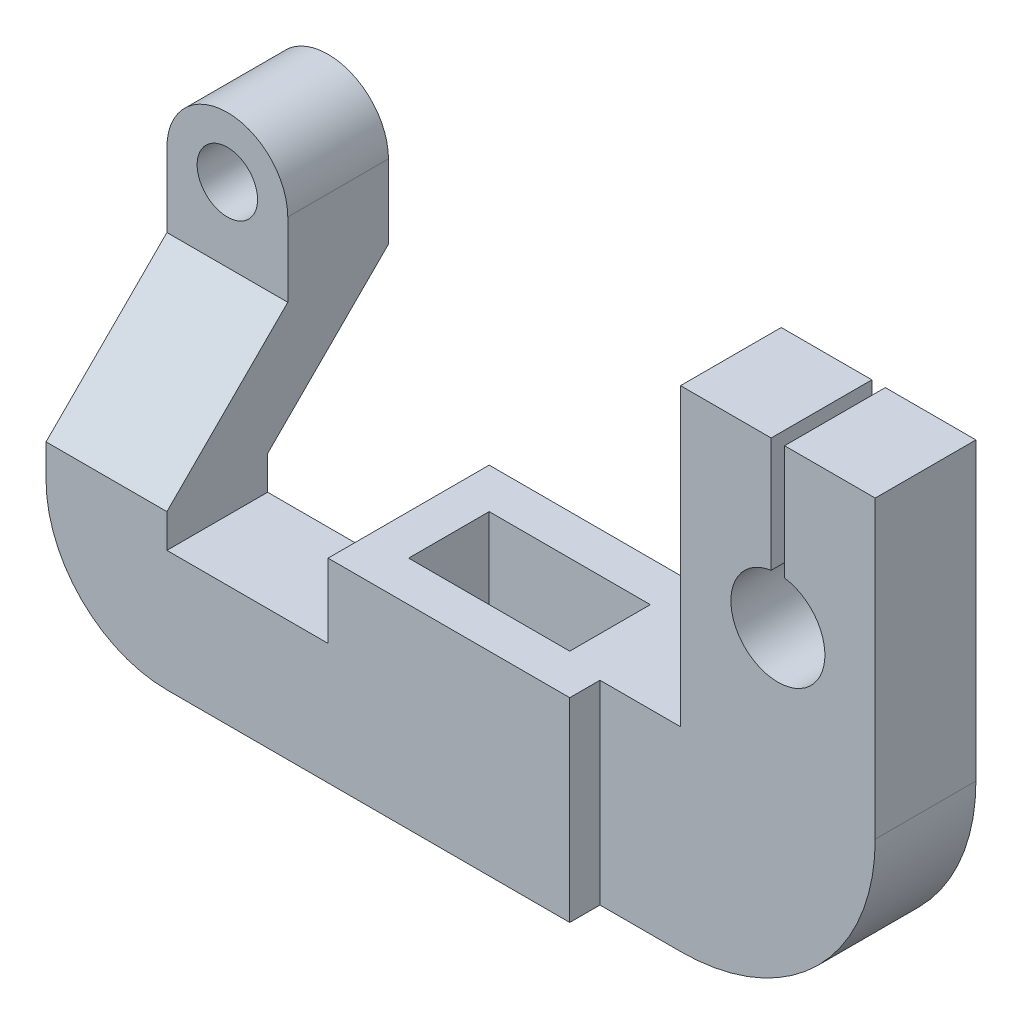
ISO-10303-21;
HEADER;
FILE_DESCRIPTION(('STEP AP214'),'2;1');
FILE_NAME('part.step','',(''),(''),'','','');
FILE_SCHEMA(('AUTOMOTIVE_DESIGN { 1 0 10303 214 1 1 1 1 }'));
ENDSEC;
DATA;
#1=APPLICATION_CONTEXT('core data for automotive mechanical design processes');
#2=APPLICATION_PROTOCOL_DEFINITION('international standard','automotive_design',2000,#1);
#3=PRODUCT_CONTEXT('',#1,'mechanical');
#4=PRODUCT('Part','Part','',(#3));
#5=PRODUCT_RELATED_PRODUCT_CATEGORY('part','',(#4));
#6=PRODUCT_DEFINITION_FORMATION('','',#4);
#7=PRODUCT_DEFINITION_CONTEXT('part definition',#1,'design');
#8=PRODUCT_DEFINITION('design','',#6,#7);
#9=PRODUCT_DEFINITION_SHAPE('','',#8);
#10=(LENGTH_UNIT() NAMED_UNIT(*) SI_UNIT(.MILLI.,.METRE.));
#11=(NAMED_UNIT(*) PLANE_ANGLE_UNIT() SI_UNIT($,.RADIAN.));
#12=(NAMED_UNIT(*) SI_UNIT($,.STERADIAN.) SOLID_ANGLE_UNIT());
#13=UNCERTAINTY_MEASURE_WITH_UNIT(LENGTH_MEASURE(1.E-05),#10,'distance_accuracy_value','');
#14=(GEOMETRIC_REPRESENTATION_CONTEXT(3) GLOBAL_UNCERTAINTY_ASSIGNED_CONTEXT((#13)) GLOBAL_UNIT_ASSIGNED_CONTEXT((#10,
#11,#12)) REPRESENTATION_CONTEXT('',''));
#15=CARTESIAN_POINT('',(0.,0.,0.));
#16=DIRECTION('',(0.,0.,1.));
#17=DIRECTION('',(1.,0.,0.));
#18=AXIS2_PLACEMENT_3D('',#15,#16,#17);
#19=CARTESIAN_POINT('',(72.,55.,-4.5));
#20=DIRECTION('',(0.,1.,0.));
#21=DIRECTION('',(0.,0.,1.));
#22=AXIS2_PLACEMENT_3D('',#19,#20,#21);
#23=PLANE('',#22);
#24=DIRECTION('',(0.,0.,-1.));
#25=VECTOR('',#24,1.);
#26=CARTESIAN_POINT('',(87.5,55.,10.5));
#27=LINE('',#26,#25);
#28=CARTESIAN_POINT('',(87.5,55.,10.5));
#29=VERTEX_POINT('',#28);
#30=CARTESIAN_POINT('',(87.5,55.,-4.5));
#31=VERTEX_POINT('',#30);
#32=EDGE_CURVE('E279',#29,#31,#27,.T.);
#33=ORIENTED_EDGE('',*,*,#32,.F.);
#34=DIRECTION('',(-1.,0.,0.));
#35=VECTOR('',#34,1.);
#36=CARTESIAN_POINT('',(72.,55.,10.5));
#37=LINE('',#36,#35);
#38=CARTESIAN_POINT('',(101.,55.,10.5));
#39=VERTEX_POINT('',#38);
#40=EDGE_CURVE('E315',#39,#29,#37,.T.);
#41=ORIENTED_EDGE('',*,*,#40,.F.);
#42=DIRECTION('',(0.,0.,1.));
#43=VECTOR('',#42,1.);
#44=CARTESIAN_POINT('',(101.,55.,-4.5));
#45=LINE('',#44,#43);
#46=CARTESIAN_POINT('',(101.,55.,-4.5));
#47=VERTEX_POINT('',#46);
#48=EDGE_CURVE('E308',#47,#39,#45,.T.);
#49=ORIENTED_EDGE('',*,*,#48,.F.);
#50=DIRECTION('',(-1.,0.,0.));
#51=VECTOR('',#50,1.);
#52=CARTESIAN_POINT('',(72.,55.,-4.5));
#53=LINE('',#52,#51);
#54=EDGE_CURVE('E305',#47,#31,#53,.T.);
#55=ORIENTED_EDGE('',*,*,#54,.T.);
#56=EDGE_LOOP('',(#33,#41,#49,#55));
#57=FACE_BOUND('',#56,.T.);
#58=ADVANCED_FACE('F44',(#57),#23,.T.);
#59=CARTESIAN_POINT('',(24.,11.,15.));
#60=DIRECTION('',(0.,-1.,0.));
#61=DIRECTION('',(0.,0.,-1.));
#62=AXIS2_PLACEMENT_3D('',#59,#60,#61);
#63=PLANE('',#62);
#64=DIRECTION('',(1.,0.,0.));
#65=VECTOR('',#64,1.);
#66=CARTESIAN_POINT('',(30.,11.,9.));
#67=LINE('',#66,#65);
#68=CARTESIAN_POINT('',(30.,11.,9.));
#69=VERTEX_POINT('',#68);
#70=CARTESIAN_POINT('',(54.,11.,9.));
#71=VERTEX_POINT('',#70);
#72=EDGE_CURVE('E268',#69,#71,#67,.T.);
#73=ORIENTED_EDGE('',*,*,#72,.F.);
#74=DIRECTION('',(0.,0.,1.));
#75=VECTOR('',#74,1.);
#76=CARTESIAN_POINT('',(30.,11.,-3.));
#77=LINE('',#76,#75);
#78=CARTESIAN_POINT('',(30.,11.,-3.));
#79=VERTEX_POINT('',#78);
#80=EDGE_CURVE('E61',#79,#69,#77,.T.);
#81=ORIENTED_EDGE('',*,*,#80,.F.);
#82=DIRECTION('',(-1.,0.,0.));
#83=VECTOR('',#82,1.);
#84=CARTESIAN_POINT('',(30.,11.,-3.));
#85=LINE('',#84,#83);
#86=CARTESIAN_POINT('',(54.,11.,-3.));
#87=VERTEX_POINT('',#86);
#88=EDGE_CURVE('E260',#87,#79,#85,.T.);
#89=ORIENTED_EDGE('',*,*,#88,.F.);
#90=DIRECTION('',(0.,0.,-1.));
#91=VECTOR('',#90,1.);
#92=CARTESIAN_POINT('',(54.,11.,-3.));
#93=LINE('',#92,#91);
#94=EDGE_CURVE('E259',#71,#87,#93,.T.);
#95=ORIENTED_EDGE('',*,*,#94,.F.);
#96=EDGE_LOOP('',(#73,#81,#89,#95));
#97=FACE_BOUND('',#96,.T.);
#98=DIRECTION('',(0.,0.,1.));
#99=VECTOR('',#98,1.);
#100=CARTESIAN_POINT('',(72.,11.,-4.5));
#101=LINE('',#100,#99);
#102=CARTESIAN_POINT('',(72.,11.,-4.5));
#103=VERTEX_POINT('',#102);
#104=CARTESIAN_POINT('',(72.,11.,10.5));
#105=VERTEX_POINT('',#104);
#106=EDGE_CURVE('E320',#103,#105,#101,.T.);
#107=ORIENTED_EDGE('',*,*,#106,.F.);
#108=DIRECTION('',(-1.,0.,0.));
#109=VECTOR('',#108,1.);
#110=CARTESIAN_POINT('',(60.,11.,-4.5));
#111=LINE('',#110,#109);
#112=CARTESIAN_POINT('',(60.,11.,-4.5));
#113=VERTEX_POINT('',#112);
#114=EDGE_CURVE('E337',#103,#113,#111,.T.);
#115=ORIENTED_EDGE('',*,*,#114,.T.);
#116=DIRECTION('',(0.,0.,-1.));
#117=VECTOR('',#116,1.);
#118=CARTESIAN_POINT('',(60.,11.,15.));
#119=LINE('',#118,#117);
#120=CARTESIAN_POINT('',(60.,11.,-9.));
#121=VERTEX_POINT('',#120);
#122=EDGE_CURVE('E447',#113,#121,#119,.T.);
#123=ORIENTED_EDGE('',*,*,#122,.T.);
#124=DIRECTION('',(1.,0.,0.));
#125=VECTOR('',#124,1.);
#126=CARTESIAN_POINT('',(60.,11.,-9.));
#127=LINE('',#126,#125);
#128=CARTESIAN_POINT('',(24.,11.,-9.));
#129=VERTEX_POINT('',#128);
#130=EDGE_CURVE('E356',#129,#121,#127,.T.);
#131=ORIENTED_EDGE('',*,*,#130,.F.);
#132=DIRECTION('',(0.,0.,-1.));
#133=VECTOR('',#132,1.);
#134=CARTESIAN_POINT('',(24.,11.,15.));
#135=LINE('',#134,#133);
#136=CARTESIAN_POINT('',(24.,11.,15.));
#137=VERTEX_POINT('',#136);
#138=EDGE_CURVE('E443',#137,#129,#135,.T.);
#139=ORIENTED_EDGE('',*,*,#138,.F.);
#140=DIRECTION('',(-1.,0.,0.));
#141=VECTOR('',#140,1.);
#142=CARTESIAN_POINT('',(24.,11.,15.));
#143=LINE('',#142,#141);
#144=CARTESIAN_POINT('',(60.,11.,15.));
#145=VERTEX_POINT('',#144);
#146=EDGE_CURVE('E425',#145,#137,#143,.T.);
#147=ORIENTED_EDGE('',*,*,#146,.F.);
#148=CARTESIAN_POINT('',(60.,11.,10.5));
#149=VERTEX_POINT('',#148);
#150=EDGE_CURVE('E450',#145,#149,#119,.T.);
#151=ORIENTED_EDGE('',*,*,#150,.T.);
#152=DIRECTION('',(1.,0.,0.));
#153=VECTOR('',#152,1.);
#154=CARTESIAN_POINT('',(72.,11.,10.5));
#155=LINE('',#154,#153);
#156=EDGE_CURVE('E333',#149,#105,#155,.T.);
#157=ORIENTED_EDGE('',*,*,#156,.T.);
#158=EDGE_LOOP('',(#107,#115,#123,#131,#139,#147,#151,#157));
#159=FACE_BOUND('',#158,.T.);
#160=ADVANCED_FACE('F530',(#97,#159),#63,.F.);
#161=CARTESIAN_POINT('',(60.,-18.,15.));
#162=DIRECTION('',(-1.,0.,0.));
#163=DIRECTION('',(0.,0.,1.));
#164=AXIS2_PLACEMENT_3D('',#161,#162,#163);
#165=PLANE('',#164);
#166=DIRECTION('',(0.,1.,0.));
#167=VECTOR('',#166,1.);
#168=CARTESIAN_POINT('',(60.,-18.,-4.5));
#169=LINE('',#168,#167);
#170=CARTESIAN_POINT('',(60.,-18.,-4.5));
#171=VERTEX_POINT('',#170);
#172=EDGE_CURVE('E343',#171,#113,#169,.T.);
#173=ORIENTED_EDGE('',*,*,#172,.F.);
#174=DIRECTION('',(0.,0.,-1.));
#175=VECTOR('',#174,1.);
#176=CARTESIAN_POINT('',(60.,-18.,15.));
#177=LINE('',#176,#175);
#178=CARTESIAN_POINT('',(60.,-18.,-9.));
#179=VERTEX_POINT('',#178);
#180=EDGE_CURVE('E448',#171,#179,#177,.T.);
#181=ORIENTED_EDGE('',*,*,#180,.T.);
#182=DIRECTION('',(0.,-1.,0.));
#183=VECTOR('',#182,1.);
#184=CARTESIAN_POINT('',(60.,-18.,-9.));
#185=LINE('',#184,#183);
#186=EDGE_CURVE('E350',#121,#179,#185,.T.);
#187=ORIENTED_EDGE('',*,*,#186,.F.);
#188=ORIENTED_EDGE('',*,*,#122,.F.);
#189=EDGE_LOOP('',(#173,#181,#187,#188));
#190=FACE_BOUND('',#189,.T.);
#191=ADVANCED_FACE('F535',(#190),#165,.F.);
#192=CARTESIAN_POINT('',(0.,0.,0.));
#193=DIRECTION('',(0.,0.,1.));
#194=DIRECTION('',(1.,0.,0.));
#195=AXIS2_PLACEMENT_3D('',#192,#193,#194);
#196=PLANE('',#195);
#197=DIRECTION('',(0.,1.,0.));
#198=VECTOR('',#197,1.);
#199=CARTESIAN_POINT('',(24.,11.,0.));
#200=LINE('',#199,#198);
#201=CARTESIAN_POINT('',(24.,-18.,0.));
#202=VERTEX_POINT('',#201);
#203=CARTESIAN_POINT('',(24.,0.,0.));
#204=VERTEX_POINT('',#203);
#205=EDGE_CURVE('E347',#202,#204,#200,.T.);
#206=ORIENTED_EDGE('',*,*,#205,.F.);
#207=DIRECTION('',(1.,0.,0.));
#208=VECTOR('',#207,1.);
#209=CARTESIAN_POINT('',(0.,-18.,0.));
#210=LINE('',#209,#208);
#211=CARTESIAN_POINT('',(0.,-18.,0.));
#212=VERTEX_POINT('',#211);
#213=EDGE_CURVE('E412',#212,#202,#210,.T.);
#214=ORIENTED_EDGE('',*,*,#213,.F.);
#215=CARTESIAN_POINT('',(0.,0.,0.));
#216=DIRECTION('',(0.,0.,1.));
#217=DIRECTION('',(1.,0.,0.));
#218=AXIS2_PLACEMENT_3D('',#215,#216,#217);
#219=CIRCLE('',#218,18.);
#220=CARTESIAN_POINT('',(-18.,0.,0.));
#221=VERTEX_POINT('',#220);
#222=EDGE_CURVE('E438',#221,#212,#219,.T.);
#223=ORIENTED_EDGE('',*,*,#222,.F.);
#224=DIRECTION('',(0.,-1.,0.));
#225=VECTOR('',#224,1.);
#226=CARTESIAN_POINT('',(-18.,0.,0.));
#227=LINE('',#226,#225);
#228=CARTESIAN_POINT('',(-18.,5.,0.));
#229=VERTEX_POINT('',#228);
#230=EDGE_CURVE('E436',#229,#221,#227,.T.);
#231=ORIENTED_EDGE('',*,*,#230,.F.);
#232=DIRECTION('',(-1.,0.,0.));
#233=VECTOR('',#232,1.);
#234=CARTESIAN_POINT('',(-18.,5.,0.));
#235=LINE('',#234,#233);
#236=CARTESIAN_POINT('',(0.,5.,0.));
#237=VERTEX_POINT('',#236);
#238=EDGE_CURVE('E433',#237,#229,#235,.T.);
#239=ORIENTED_EDGE('',*,*,#238,.F.);
#240=DIRECTION('',(0.,1.,0.));
#241=VECTOR('',#240,1.);
#242=CARTESIAN_POINT('',(0.,5.,0.));
#243=LINE('',#242,#241);
#244=CARTESIAN_POINT('',(0.,0.,0.));
#245=VERTEX_POINT('',#244);
#246=EDGE_CURVE('E431',#245,#237,#243,.T.);
#247=ORIENTED_EDGE('',*,*,#246,.F.);
#248=DIRECTION('',(-1.,0.,0.));
#249=VECTOR('',#248,1.);
#250=CARTESIAN_POINT('',(0.,0.,0.));
#251=LINE('',#250,#249);
#252=EDGE_CURVE('E406',#204,#245,#251,.T.);
#253=ORIENTED_EDGE('',*,*,#252,.F.);
#254=EDGE_LOOP('',(#206,#214,#223,#231,#239,#247,#253));
#255=FACE_BOUND('',#254,.T.);
#256=ADVANCED_FACE('F509',(#255),#196,.F.);
#257=CARTESIAN_POINT('',(0.,0.,15.));
#258=DIRECTION('',(0.,-1.,0.));
#259=DIRECTION('',(0.,0.,-1.));
#260=AXIS2_PLACEMENT_3D('',#257,#258,#259);
#261=PLANE('',#260);
#262=ORIENTED_EDGE('',*,*,#252,.T.);
#263=DIRECTION('',(0.,0.,-1.));
#264=VECTOR('',#263,1.);
#265=CARTESIAN_POINT('',(0.,0.,15.));
#266=LINE('',#265,#264);
#267=CARTESIAN_POINT('',(0.,0.,15.));
#268=VERTEX_POINT('',#267);
#269=EDGE_CURVE('E460',#268,#245,#266,.T.);
#270=ORIENTED_EDGE('',*,*,#269,.F.);
#271=DIRECTION('',(-1.,0.,0.));
#272=VECTOR('',#271,1.);
#273=CARTESIAN_POINT('',(0.,0.,15.));
#274=LINE('',#273,#272);
#275=CARTESIAN_POINT('',(24.,0.,15.));
#276=VERTEX_POINT('',#275);
#277=EDGE_CURVE('E407',#276,#268,#274,.T.);
#278=ORIENTED_EDGE('',*,*,#277,.F.);
#279=DIRECTION('',(0.,0.,-1.));
#280=VECTOR('',#279,1.);
#281=CARTESIAN_POINT('',(24.,0.,15.));
#282=LINE('',#281,#280);
#283=EDGE_CURVE('E426',#276,#204,#282,.T.);
#284=ORIENTED_EDGE('',*,*,#283,.T.);
#285=EDGE_LOOP('',(#262,#270,#278,#284));
#286=FACE_BOUND('',#285,.T.);
#287=ADVANCED_FACE('F50',(#286),#261,.F.);
#288=CARTESIAN_POINT('',(0.,5.,15.));
#289=DIRECTION('',(-1.,0.,0.));
#290=DIRECTION('',(0.,0.,1.));
#291=AXIS2_PLACEMENT_3D('',#288,#289,#290);
#292=PLANE('',#291);
#293=ORIENTED_EDGE('',*,*,#246,.T.);
#294=DIRECTION('',(0.,-0.707106781186547,0.707106781186548));
#295=VECTOR('',#294,1.);
#296=CARTESIAN_POINT('',(0.,5.,0.));
#297=LINE('',#296,#295);
#298=CARTESIAN_POINT('',(0.,23.,-18.));
#299=VERTEX_POINT('',#298);
#300=EDGE_CURVE('E392',#299,#237,#297,.T.);
#301=ORIENTED_EDGE('',*,*,#300,.F.);
#302=DIRECTION('',(0.,-1.,0.));
#303=VECTOR('',#302,1.);
#304=CARTESIAN_POINT('',(0.,23.,-18.));
#305=LINE('',#304,#303);
#306=CARTESIAN_POINT('',(0.,34.,-18.));
#307=VERTEX_POINT('',#306);
#308=EDGE_CURVE('E382',#307,#299,#305,.T.);
#309=ORIENTED_EDGE('',*,*,#308,.F.);
#310=DIRECTION('',(0.,0.,-1.));
#311=VECTOR('',#310,1.);
#312=CARTESIAN_POINT('',(0.,34.,-18.));
#313=LINE('',#312,#311);
#314=CARTESIAN_POINT('',(0.,34.,-3.));
#315=VERTEX_POINT('',#314);
#316=EDGE_CURVE('E377',#315,#307,#313,.T.);
#317=ORIENTED_EDGE('',*,*,#316,.F.);
#318=DIRECTION('',(0.,1.,0.));
#319=VECTOR('',#318,1.);
#320=CARTESIAN_POINT('',(0.,34.,-3.));
#321=LINE('',#320,#319);
#322=CARTESIAN_POINT('',(0.,23.,-3.));
#323=VERTEX_POINT('',#322);
#324=EDGE_CURVE('E374',#323,#315,#321,.T.);
#325=ORIENTED_EDGE('',*,*,#324,.F.);
#326=DIRECTION('',(0.,0.707106781186547,-0.707106781186548));
#327=VECTOR('',#326,1.);
#328=CARTESIAN_POINT('',(0.,23.,-3.));
#329=LINE('',#328,#327);
#330=CARTESIAN_POINT('',(0.,5.,15.));
#331=VERTEX_POINT('',#330);
#332=EDGE_CURVE('E395',#331,#323,#329,.T.);
#333=ORIENTED_EDGE('',*,*,#332,.F.);
#334=DIRECTION('',(0.,1.,0.));
#335=VECTOR('',#334,1.);
#336=CARTESIAN_POINT('',(0.,5.,15.));
#337=LINE('',#336,#335);
#338=EDGE_CURVE('E411',#268,#331,#337,.T.);
#339=ORIENTED_EDGE('',*,*,#338,.F.);
#340=ORIENTED_EDGE('',*,*,#269,.T.);
#341=EDGE_LOOP('',(#293,#301,#309,#317,#325,#333,#339,#340));
#342=FACE_BOUND('',#341,.T.);
#343=ADVANCED_FACE('F759',(#342),#292,.F.);
#344=CARTESIAN_POINT('',(-18.,0.,15.));
#345=DIRECTION('',(1.,0.,0.));
#346=DIRECTION('',(0.,0.,-1.));
#347=AXIS2_PLACEMENT_3D('',#344,#345,#346);
#348=PLANE('',#347);
#349=ORIENTED_EDGE('',*,*,#230,.T.);
#350=DIRECTION('',(0.,0.,-1.));
#351=VECTOR('',#350,1.);
#352=CARTESIAN_POINT('',(-18.,0.,15.));
#353=LINE('',#352,#351);
#354=CARTESIAN_POINT('',(-18.,0.,15.));
#355=VERTEX_POINT('',#354);
#356=EDGE_CURVE('E457',#355,#221,#353,.T.);
#357=ORIENTED_EDGE('',*,*,#356,.F.);
#358=DIRECTION('',(0.,-1.,0.));
#359=VECTOR('',#358,1.);
#360=CARTESIAN_POINT('',(-18.,0.,15.));
#361=LINE('',#360,#359);
#362=CARTESIAN_POINT('',(-18.,5.,15.));
#363=VERTEX_POINT('',#362);
#364=EDGE_CURVE('E418',#363,#355,#361,.T.);
#365=ORIENTED_EDGE('',*,*,#364,.F.);
#366=DIRECTION('',(0.,0.707106781186547,-0.707106781186548));
#367=VECTOR('',#366,1.);
#368=CARTESIAN_POINT('',(-18.,23.,-3.));
#369=LINE('',#368,#367);
#370=CARTESIAN_POINT('',(-18.,23.,-3.));
#371=VERTEX_POINT('',#370);
#372=EDGE_CURVE('E398',#363,#371,#369,.T.);
#373=ORIENTED_EDGE('',*,*,#372,.T.);
#374=DIRECTION('',(0.,1.,0.));
#375=VECTOR('',#374,1.);
#376=CARTESIAN_POINT('',(-18.,34.,-3.));
#377=LINE('',#376,#375);
#378=CARTESIAN_POINT('',(-18.,34.,-3.));
#379=VERTEX_POINT('',#378);
#380=EDGE_CURVE('E373',#371,#379,#377,.T.);
#381=ORIENTED_EDGE('',*,*,#380,.T.);
#382=DIRECTION('',(0.,0.,-1.));
#383=VECTOR('',#382,1.);
#384=CARTESIAN_POINT('',(-18.,34.,-18.));
#385=LINE('',#384,#383);
#386=CARTESIAN_POINT('',(-18.,34.,-18.));
#387=VERTEX_POINT('',#386);
#388=EDGE_CURVE('E390',#379,#387,#385,.T.);
#389=ORIENTED_EDGE('',*,*,#388,.T.);
#390=DIRECTION('',(0.,-1.,0.));
#391=VECTOR('',#390,1.);
#392=CARTESIAN_POINT('',(-18.,23.,-18.));
#393=LINE('',#392,#391);
#394=CARTESIAN_POINT('',(-18.,23.,-18.));
#395=VERTEX_POINT('',#394);
#396=EDGE_CURVE('E378',#387,#395,#393,.T.);
#397=ORIENTED_EDGE('',*,*,#396,.T.);
#398=DIRECTION('',(0.,-0.707106781186547,0.707106781186548));
#399=VECTOR('',#398,1.);
#400=CARTESIAN_POINT('',(-18.,5.,0.));
#401=LINE('',#400,#399);
#402=EDGE_CURVE('E381',#395,#229,#401,.T.);
#403=ORIENTED_EDGE('',*,*,#402,.T.);
#404=EDGE_LOOP('',(#349,#357,#365,#373,#381,#389,#397,#403));
#405=FACE_BOUND('',#404,.T.);
#406=ADVANCED_FACE('F753',(#405),#348,.F.);
#407=CARTESIAN_POINT('',(0.,0.,15.));
#408=DIRECTION('',(0.,0.,-1.));
#409=DIRECTION('',(-1.,0.,0.));
#410=AXIS2_PLACEMENT_3D('',#407,#408,#409);
#411=CYLINDRICAL_SURFACE('',#410,18.);
#412=ORIENTED_EDGE('',*,*,#222,.T.);
#413=DIRECTION('',(0.,0.,-1.));
#414=VECTOR('',#413,1.);
#415=CARTESIAN_POINT('',(0.,-18.,15.));
#416=LINE('',#415,#414);
#417=CARTESIAN_POINT('',(0.,-18.,15.));
#418=VERTEX_POINT('',#417);
#419=EDGE_CURVE('E453',#418,#212,#416,.T.);
#420=ORIENTED_EDGE('',*,*,#419,.F.);
#421=CARTESIAN_POINT('',(0.,0.,15.));
#422=DIRECTION('',(0.,0.,1.));
#423=DIRECTION('',(1.,0.,0.));
#424=AXIS2_PLACEMENT_3D('',#421,#422,#423);
#425=CIRCLE('',#424,18.);
#426=EDGE_CURVE('E416',#355,#418,#425,.T.);
#427=ORIENTED_EDGE('',*,*,#426,.F.);
#428=ORIENTED_EDGE('',*,*,#356,.T.);
#429=EDGE_LOOP('',(#412,#420,#427,#428));
#430=FACE_BOUND('',#429,.T.);
#431=ADVANCED_FACE('F743',(#430),#411,.T.);
#432=CARTESIAN_POINT('',(0.,-18.,15.));
#433=DIRECTION('',(0.,1.,0.));
#434=DIRECTION('',(0.,0.,1.));
#435=AXIS2_PLACEMENT_3D('',#432,#433,#434);
#436=PLANE('',#435);
#437=ORIENTED_EDGE('',*,*,#213,.T.);
#438=DIRECTION('',(0.,0.,1.));
#439=VECTOR('',#438,1.);
#440=CARTESIAN_POINT('',(24.,-18.,-9.));
#441=LINE('',#440,#439);
#442=CARTESIAN_POINT('',(24.,-18.,-9.));
#443=VERTEX_POINT('',#442);
#444=EDGE_CURVE('E363',#443,#202,#441,.T.);
#445=ORIENTED_EDGE('',*,*,#444,.F.);
#446=DIRECTION('',(-1.,0.,0.));
#447=VECTOR('',#446,1.);
#448=CARTESIAN_POINT('',(24.,-18.,-9.));
#449=LINE('',#448,#447);
#450=EDGE_CURVE('E351',#179,#443,#449,.T.);
#451=ORIENTED_EDGE('',*,*,#450,.F.);
#452=ORIENTED_EDGE('',*,*,#180,.F.);
#453=DIRECTION('',(-1.,0.,0.));
#454=VECTOR('',#453,1.);
#455=CARTESIAN_POINT('',(60.,-18.,-4.5));
#456=LINE('',#455,#454);
#457=CARTESIAN_POINT('',(72.,-18.,-4.5));
#458=VERTEX_POINT('',#457);
#459=EDGE_CURVE('E339',#458,#171,#456,.T.);
#460=ORIENTED_EDGE('',*,*,#459,.F.);
#461=DIRECTION('',(0.,0.,-1.));
#462=VECTOR('',#461,1.);
#463=CARTESIAN_POINT('',(72.,-18.,-4.5));
#464=LINE('',#463,#462);
#465=CARTESIAN_POINT('',(72.,-18.,10.5));
#466=VERTEX_POINT('',#465);
#467=EDGE_CURVE('E332',#466,#458,#464,.T.);
#468=ORIENTED_EDGE('',*,*,#467,.F.);
#469=DIRECTION('',(1.,0.,0.));
#470=VECTOR('',#469,1.);
#471=CARTESIAN_POINT('',(72.,-18.,10.5));
#472=LINE('',#471,#470);
#473=CARTESIAN_POINT('',(60.,-18.,10.5));
#474=VERTEX_POINT('',#473);
#475=EDGE_CURVE('E335',#474,#466,#472,.T.);
#476=ORIENTED_EDGE('',*,*,#475,.F.);
#477=CARTESIAN_POINT('',(60.,-18.,15.));
#478=VERTEX_POINT('',#477);
#479=EDGE_CURVE('E451',#478,#474,#177,.T.);
#480=ORIENTED_EDGE('',*,*,#479,.F.);
#481=DIRECTION('',(1.,0.,0.));
#482=VECTOR('',#481,1.);
#483=CARTESIAN_POINT('',(0.,-18.,15.));
#484=LINE('',#483,#482);
#485=EDGE_CURVE('E417',#418,#478,#484,.T.);
#486=ORIENTED_EDGE('',*,*,#485,.F.);
#487=ORIENTED_EDGE('',*,*,#419,.T.);
#488=EDGE_LOOP('',(#437,#445,#451,#452,#460,#468,#476,#480,#486,#487));
#489=FACE_BOUND('',#488,.T.);
#490=ADVANCED_FACE('F495',(#489),#436,.F.);
#491=ORIENTED_EDGE('',*,*,#479,.T.);
#492=DIRECTION('',(0.,1.,0.));
#493=VECTOR('',#492,1.);
#494=CARTESIAN_POINT('',(60.,-18.,10.5));
#495=LINE('',#494,#493);
#496=EDGE_CURVE('E341',#474,#149,#495,.T.);
#497=ORIENTED_EDGE('',*,*,#496,.T.);
#498=ORIENTED_EDGE('',*,*,#150,.F.);
#499=DIRECTION('',(0.,1.,0.));
#500=VECTOR('',#499,1.);
#501=CARTESIAN_POINT('',(60.,-18.,15.));
#502=LINE('',#501,#500);
#503=EDGE_CURVE('E422',#478,#145,#502,.T.);
#504=ORIENTED_EDGE('',*,*,#503,.F.);
#505=EDGE_LOOP('',(#491,#497,#498,#504));
#506=FACE_BOUND('',#505,.T.);
#507=ADVANCED_FACE('F496',(#506),#165,.F.);
#508=CARTESIAN_POINT('',(24.,0.,15.));
#509=DIRECTION('',(1.,0.,0.));
#510=DIRECTION('',(0.,0.,-1.));
#511=AXIS2_PLACEMENT_3D('',#508,#509,#510);
#512=PLANE('',#511);
#513=ORIENTED_EDGE('',*,*,#138,.T.);
#514=DIRECTION('',(0.,1.,0.));
#515=VECTOR('',#514,1.);
#516=CARTESIAN_POINT('',(24.,11.,-9.));
#517=LINE('',#516,#515);
#518=EDGE_CURVE('E352',#443,#129,#517,.T.);
#519=ORIENTED_EDGE('',*,*,#518,.F.);
#520=ORIENTED_EDGE('',*,*,#444,.T.);
#521=ORIENTED_EDGE('',*,*,#205,.T.);
#522=ORIENTED_EDGE('',*,*,#283,.F.);
#523=DIRECTION('',(0.,-1.,0.));
#524=VECTOR('',#523,1.);
#525=CARTESIAN_POINT('',(24.,0.,15.));
#526=LINE('',#525,#524);
#527=EDGE_CURVE('E428',#137,#276,#526,.T.);
#528=ORIENTED_EDGE('',*,*,#527,.F.);
#529=EDGE_LOOP('',(#513,#519,#520,#521,#522,#528));
#530=FACE_BOUND('',#529,.T.);
#531=ADVANCED_FACE('F511',(#530),#512,.F.);
#532=CARTESIAN_POINT('',(0.,0.,15.));
#533=DIRECTION('',(0.,0.,1.));
#534=DIRECTION('',(1.,0.,0.));
#535=AXIS2_PLACEMENT_3D('',#532,#533,#534);
#536=PLANE('',#535);
#537=ORIENTED_EDGE('',*,*,#277,.T.);
#538=ORIENTED_EDGE('',*,*,#338,.T.);
#539=DIRECTION('',(-1.,0.,0.));
#540=VECTOR('',#539,1.);
#541=CARTESIAN_POINT('',(-18.,5.,15.));
#542=LINE('',#541,#540);
#543=EDGE_CURVE('E413',#331,#363,#542,.T.);
#544=ORIENTED_EDGE('',*,*,#543,.T.);
#545=ORIENTED_EDGE('',*,*,#364,.T.);
#546=ORIENTED_EDGE('',*,*,#426,.T.);
#547=ORIENTED_EDGE('',*,*,#485,.T.);
#548=ORIENTED_EDGE('',*,*,#503,.T.);
#549=ORIENTED_EDGE('',*,*,#146,.T.);
#550=ORIENTED_EDGE('',*,*,#527,.T.);
#551=EDGE_LOOP('',(#537,#538,#544,#545,#546,#547,#548,#549,#550));
#552=FACE_BOUND('',#551,.T.);
#553=ADVANCED_FACE('F499',(#552),#536,.T.);
#554=CARTESIAN_POINT('',(0.,5.,0.));
#555=DIRECTION('',(0.,-0.707106781186548,-0.707106781186547));
#556=DIRECTION('',(0.,0.707106781186547,-0.707106781186548));
#557=AXIS2_PLACEMENT_3D('',#554,#555,#556);
#558=PLANE('',#557);
#559=ORIENTED_EDGE('',*,*,#402,.F.);
#560=DIRECTION('',(-1.,0.,0.));
#561=VECTOR('',#560,1.);
#562=CARTESIAN_POINT('',(0.,23.,-18.));
#563=LINE('',#562,#561);
#564=EDGE_CURVE('E401',#299,#395,#563,.T.);
#565=ORIENTED_EDGE('',*,*,#564,.F.);
#566=ORIENTED_EDGE('',*,*,#300,.T.);
#567=ORIENTED_EDGE('',*,*,#238,.T.);
#568=EDGE_LOOP('',(#559,#565,#566,#567));
#569=FACE_BOUND('',#568,.T.);
#570=ADVANCED_FACE('F703',(#569),#558,.T.);
#571=CARTESIAN_POINT('',(0.,23.,-3.));
#572=DIRECTION('',(0.,0.707106781186548,0.707106781186547));
#573=DIRECTION('',(0.,-0.707106781186547,0.707106781186548));
#574=AXIS2_PLACEMENT_3D('',#571,#572,#573);
#575=PLANE('',#574);
#576=ORIENTED_EDGE('',*,*,#372,.F.);
#577=ORIENTED_EDGE('',*,*,#543,.F.);
#578=ORIENTED_EDGE('',*,*,#332,.T.);
#579=DIRECTION('',(-1.,0.,0.));
#580=VECTOR('',#579,1.);
#581=CARTESIAN_POINT('',(0.,23.,-3.));
#582=LINE('',#581,#580);
#583=EDGE_CURVE('E396',#323,#371,#582,.T.);
#584=ORIENTED_EDGE('',*,*,#583,.T.);
#585=EDGE_LOOP('',(#576,#577,#578,#584));
#586=FACE_BOUND('',#585,.T.);
#587=ADVANCED_FACE('F692',(#586),#575,.T.);
#588=CARTESIAN_POINT('',(0.,23.,-18.));
#589=DIRECTION('',(0.,0.,-1.));
#590=DIRECTION('',(-1.,0.,0.));
#591=AXIS2_PLACEMENT_3D('',#588,#589,#590);
#592=PLANE('',#591);
#593=CARTESIAN_POINT('',(-9.,34.,-18.));
#594=DIRECTION('',(0.,0.,1.));
#595=DIRECTION('',(1.,0.,0.));
#596=AXIS2_PLACEMENT_3D('',#593,#594,#595);
#597=CIRCLE('',#596,4.5);
#598=CARTESIAN_POINT('',(-4.5,34.,-18.));
#599=VERTEX_POINT('',#598);
#600=EDGE_CURVE('E362',#599,#599,#597,.T.);
#601=ORIENTED_EDGE('',*,*,#600,.T.);
#602=EDGE_LOOP('',(#601));
#603=FACE_BOUND('',#602,.T.);
#604=ORIENTED_EDGE('',*,*,#396,.F.);
#605=CARTESIAN_POINT('',(-9.,34.,-18.));
#606=DIRECTION('',(0.,0.,1.));
#607=DIRECTION('',(1.,0.,0.));
#608=AXIS2_PLACEMENT_3D('',#605,#606,#607);
#609=CIRCLE('',#608,9.);
#610=EDGE_CURVE('E371',#307,#387,#609,.T.);
#611=ORIENTED_EDGE('',*,*,#610,.F.);
#612=ORIENTED_EDGE('',*,*,#308,.T.);
#613=ORIENTED_EDGE('',*,*,#564,.T.);
#614=EDGE_LOOP('',(#604,#611,#612,#613));
#615=FACE_BOUND('',#614,.T.);
#616=ADVANCED_FACE('F684',(#603,#615),#592,.T.);
#617=CARTESIAN_POINT('',(0.,34.,-3.));
#618=DIRECTION('',(0.,0.,1.));
#619=DIRECTION('',(0.,-1.,0.));
#620=AXIS2_PLACEMENT_3D('',#617,#618,#619);
#621=PLANE('',#620);
#622=CARTESIAN_POINT('',(-9.,34.,-3.));
#623=DIRECTION('',(0.,0.,1.));
#624=DIRECTION('',(1.,0.,0.));
#625=AXIS2_PLACEMENT_3D('',#622,#623,#624);
#626=CIRCLE('',#625,4.5);
#627=CARTESIAN_POINT('',(-4.5,34.,-3.));
#628=VERTEX_POINT('',#627);
#629=EDGE_CURVE('E364',#628,#628,#626,.T.);
#630=ORIENTED_EDGE('',*,*,#629,.F.);
#631=EDGE_LOOP('',(#630));
#632=FACE_BOUND('',#631,.T.);
#633=ORIENTED_EDGE('',*,*,#380,.F.);
#634=ORIENTED_EDGE('',*,*,#583,.F.);
#635=ORIENTED_EDGE('',*,*,#324,.T.);
#636=CARTESIAN_POINT('',(-9.,34.,-3.));
#637=DIRECTION('',(0.,0.,1.));
#638=DIRECTION('',(1.,0.,0.));
#639=AXIS2_PLACEMENT_3D('',#636,#637,#638);
#640=CIRCLE('',#639,9.);
#641=EDGE_CURVE('E368',#315,#379,#640,.T.);
#642=ORIENTED_EDGE('',*,*,#641,.T.);
#643=EDGE_LOOP('',(#633,#634,#635,#642));
#644=FACE_BOUND('',#643,.T.);
#645=ADVANCED_FACE('F674',(#632,#644),#621,.T.);
#646=CARTESIAN_POINT('',(-9.,34.,-18.));
#647=DIRECTION('',(0.,0.,1.));
#648=DIRECTION('',(1.,0.,0.));
#649=AXIS2_PLACEMENT_3D('',#646,#647,#648);
#650=CYLINDRICAL_SURFACE('',#649,9.);
#651=ORIENTED_EDGE('',*,*,#641,.F.);
#652=ORIENTED_EDGE('',*,*,#316,.T.);
#653=ORIENTED_EDGE('',*,*,#610,.T.);
#654=ORIENTED_EDGE('',*,*,#388,.F.);
#655=EDGE_LOOP('',(#651,#652,#653,#654));
#656=FACE_BOUND('',#655,.T.);
#657=ADVANCED_FACE('F662',(#656),#650,.T.);
#658=CARTESIAN_POINT('',(-9.,34.,-18.));
#659=DIRECTION('',(0.,0.,1.));
#660=DIRECTION('',(1.,0.,0.));
#661=AXIS2_PLACEMENT_3D('',#658,#659,#660);
#662=CYLINDRICAL_SURFACE('',#661,4.5);
#663=ORIENTED_EDGE('',*,*,#600,.F.);
#664=EDGE_LOOP('',(#663));
#665=FACE_BOUND('',#664,.T.);
#666=ORIENTED_EDGE('',*,*,#629,.T.);
#667=EDGE_LOOP('',(#666));
#668=FACE_BOUND('',#667,.T.);
#669=ADVANCED_FACE('F649',(#665,#668),#662,.F.);
#670=CARTESIAN_POINT('',(0.,0.,-9.));
#671=DIRECTION('',(0.,0.,1.));
#672=DIRECTION('',(1.,0.,0.));
#673=AXIS2_PLACEMENT_3D('',#670,#671,#672);
#674=PLANE('',#673);
#675=ORIENTED_EDGE('',*,*,#186,.T.);
#676=ORIENTED_EDGE('',*,*,#450,.T.);
#677=ORIENTED_EDGE('',*,*,#518,.T.);
#678=ORIENTED_EDGE('',*,*,#130,.T.);
#679=EDGE_LOOP('',(#675,#676,#677,#678));
#680=FACE_BOUND('',#679,.T.);
#681=ADVANCED_FACE('F523',(#680),#674,.F.);
#682=CARTESIAN_POINT('',(60.,-18.,-4.5));
#683=DIRECTION('',(0.,0.,-1.));
#684=DIRECTION('',(-1.,0.,0.));
#685=AXIS2_PLACEMENT_3D('',#682,#683,#684);
#686=PLANE('',#685);
#687=DIRECTION('',(0.,1.,0.));
#688=VECTOR('',#687,1.);
#689=CARTESIAN_POINT('',(87.5,37.,-4.5));
#690=LINE('',#689,#688);
#691=CARTESIAN_POINT('',(87.5,37.9282032302755,-4.5));
#692=VERTEX_POINT('',#691);
#693=EDGE_CURVE('E284',#692,#31,#690,.T.);
#694=ORIENTED_EDGE('',*,*,#693,.T.);
#695=ORIENTED_EDGE('',*,*,#54,.F.);
#696=DIRECTION('',(0.,1.,0.));
#697=VECTOR('',#696,1.);
#698=CARTESIAN_POINT('',(101.,55.,-4.5));
#699=LINE('',#698,#697);
#700=CARTESIAN_POINT('',(101.,11.,-4.5));
#701=VERTEX_POINT('',#700);
#702=EDGE_CURVE('E300',#701,#47,#699,.T.);
#703=ORIENTED_EDGE('',*,*,#702,.F.);
#704=CARTESIAN_POINT('',(72.,11.,-4.5));
#705=DIRECTION('',(0.,0.,1.));
#706=DIRECTION('',(1.,0.,0.));
#707=AXIS2_PLACEMENT_3D('',#704,#705,#706);
#708=CIRCLE('',#707,29.);
#709=EDGE_CURVE('E324',#458,#701,#708,.T.);
#710=ORIENTED_EDGE('',*,*,#709,.F.);
#711=ORIENTED_EDGE('',*,*,#459,.T.);
#712=ORIENTED_EDGE('',*,*,#172,.T.);
#713=ORIENTED_EDGE('',*,*,#114,.F.);
#714=DIRECTION('',(0.,-1.,0.));
#715=VECTOR('',#714,1.);
#716=CARTESIAN_POINT('',(72.,31.,-4.5));
#717=LINE('',#716,#715);
#718=CARTESIAN_POINT('',(72.,55.,-4.5));
#719=VERTEX_POINT('',#718);
#720=EDGE_CURVE('E304',#719,#103,#717,.T.);
#721=ORIENTED_EDGE('',*,*,#720,.F.);
#722=CARTESIAN_POINT('',(85.5,55.,-4.5));
#723=VERTEX_POINT('',#722);
#724=EDGE_CURVE('E297',#723,#719,#53,.T.);
#725=ORIENTED_EDGE('',*,*,#724,.F.);
#726=DIRECTION('',(0.,1.,0.));
#727=VECTOR('',#726,1.);
#728=CARTESIAN_POINT('',(85.5,37.,-4.5));
#729=LINE('',#728,#727);
#730=CARTESIAN_POINT('',(85.5,37.9282032302755,-4.5));
#731=VERTEX_POINT('',#730);
#732=EDGE_CURVE('E282',#731,#723,#729,.T.);
#733=ORIENTED_EDGE('',*,*,#732,.F.);
#734=CARTESIAN_POINT('',(86.5,31.,-4.5));
#735=DIRECTION('',(0.,0.,1.));
#736=DIRECTION('',(1.,0.,0.));
#737=AXIS2_PLACEMENT_3D('',#734,#735,#736);
#738=CIRCLE('',#737,7.);
#739=EDGE_CURVE('E293',#731,#692,#738,.T.);
#740=ORIENTED_EDGE('',*,*,#739,.T.);
#741=EDGE_LOOP('',(#694,#695,#703,#710,#711,#712,#713,#721,#725,#733,#740));
#742=FACE_BOUND('',#741,.T.);
#743=ADVANCED_FACE('F480',(#742),#686,.T.);
#744=CARTESIAN_POINT('',(72.,-18.,10.5));
#745=DIRECTION('',(0.,0.,1.));
#746=DIRECTION('',(1.,0.,0.));
#747=AXIS2_PLACEMENT_3D('',#744,#745,#746);
#748=PLANE('',#747);
#749=DIRECTION('',(0.,1.,0.));
#750=VECTOR('',#749,1.);
#751=CARTESIAN_POINT('',(87.5,37.,10.5));
#752=LINE('',#751,#750);
#753=CARTESIAN_POINT('',(87.5,37.9282032302755,10.5));
#754=VERTEX_POINT('',#753);
#755=EDGE_CURVE('E290',#754,#29,#752,.T.);
#756=ORIENTED_EDGE('',*,*,#755,.F.);
#757=CARTESIAN_POINT('',(86.5,31.,10.5));
#758=DIRECTION('',(0.,0.,1.));
#759=DIRECTION('',(1.,0.,0.));
#760=AXIS2_PLACEMENT_3D('',#757,#758,#759);
#761=CIRCLE('',#760,7.);
#762=CARTESIAN_POINT('',(85.5,37.9282032302755,10.5));
#763=VERTEX_POINT('',#762);
#764=EDGE_CURVE('E288',#763,#754,#761,.T.);
#765=ORIENTED_EDGE('',*,*,#764,.F.);
#766=DIRECTION('',(0.,1.,0.));
#767=VECTOR('',#766,1.);
#768=CARTESIAN_POINT('',(85.5,37.,10.5));
#769=LINE('',#768,#767);
#770=CARTESIAN_POINT('',(85.5,55.,10.5));
#771=VERTEX_POINT('',#770);
#772=EDGE_CURVE('E68',#763,#771,#769,.T.);
#773=ORIENTED_EDGE('',*,*,#772,.T.);
#774=CARTESIAN_POINT('',(72.,55.,10.5));
#775=VERTEX_POINT('',#774);
#776=EDGE_CURVE('E311',#771,#775,#37,.T.);
#777=ORIENTED_EDGE('',*,*,#776,.T.);
#778=DIRECTION('',(0.,-1.,0.));
#779=VECTOR('',#778,1.);
#780=CARTESIAN_POINT('',(72.,11.,10.5));
#781=LINE('',#780,#779);
#782=EDGE_CURVE('E301',#775,#105,#781,.T.);
#783=ORIENTED_EDGE('',*,*,#782,.T.);
#784=ORIENTED_EDGE('',*,*,#156,.F.);
#785=ORIENTED_EDGE('',*,*,#496,.F.);
#786=ORIENTED_EDGE('',*,*,#475,.T.);
#787=CARTESIAN_POINT('',(72.,11.,10.5));
#788=DIRECTION('',(0.,0.,1.));
#789=DIRECTION('',(1.,0.,0.));
#790=AXIS2_PLACEMENT_3D('',#787,#788,#789);
#791=CIRCLE('',#790,29.);
#792=CARTESIAN_POINT('',(101.,11.,10.5));
#793=VERTEX_POINT('',#792);
#794=EDGE_CURVE('E318',#466,#793,#791,.T.);
#795=ORIENTED_EDGE('',*,*,#794,.T.);
#796=DIRECTION('',(0.,1.,0.));
#797=VECTOR('',#796,1.);
#798=CARTESIAN_POINT('',(101.,55.,10.5));
#799=LINE('',#798,#797);
#800=EDGE_CURVE('E295',#793,#39,#799,.T.);
#801=ORIENTED_EDGE('',*,*,#800,.T.);
#802=ORIENTED_EDGE('',*,*,#40,.T.);
#803=EDGE_LOOP('',(#756,#765,#773,#777,#783,#784,#785,#786,#795,#801,#802));
#804=FACE_BOUND('',#803,.T.);
#805=ADVANCED_FACE('F468',(#804),#748,.T.);
#806=CARTESIAN_POINT('',(72.,11.,-4.5));
#807=DIRECTION('',(0.,0.,1.));
#808=DIRECTION('',(1.,0.,0.));
#809=AXIS2_PLACEMENT_3D('',#806,#807,#808);
#810=CYLINDRICAL_SURFACE('',#809,29.);
#811=ORIENTED_EDGE('',*,*,#794,.F.);
#812=ORIENTED_EDGE('',*,*,#467,.T.);
#813=ORIENTED_EDGE('',*,*,#709,.T.);
#814=DIRECTION('',(0.,0.,1.));
#815=VECTOR('',#814,1.);
#816=CARTESIAN_POINT('',(101.,11.,-4.5));
#817=LINE('',#816,#815);
#818=EDGE_CURVE('E327',#701,#793,#817,.T.);
#819=ORIENTED_EDGE('',*,*,#818,.T.);
#820=EDGE_LOOP('',(#811,#812,#813,#819));
#821=FACE_BOUND('',#820,.T.);
#822=ADVANCED_FACE('F486',(#821),#810,.T.);
#823=CARTESIAN_POINT('',(101.,55.,-4.5));
#824=DIRECTION('',(1.,0.,0.));
#825=DIRECTION('',(0.,0.,-1.));
#826=AXIS2_PLACEMENT_3D('',#823,#824,#825);
#827=PLANE('',#826);
#828=ORIENTED_EDGE('',*,*,#800,.F.);
#829=ORIENTED_EDGE('',*,*,#818,.F.);
#830=ORIENTED_EDGE('',*,*,#702,.T.);
#831=ORIENTED_EDGE('',*,*,#48,.T.);
#832=EDGE_LOOP('',(#828,#829,#830,#831));
#833=FACE_BOUND('',#832,.T.);
#834=ADVANCED_FACE('F482',(#833),#827,.T.);
#835=CARTESIAN_POINT('',(72.,11.,-4.5));
#836=DIRECTION('',(-1.,0.,0.));
#837=DIRECTION('',(0.,0.,1.));
#838=AXIS2_PLACEMENT_3D('',#835,#836,#837);
#839=PLANE('',#838);
#840=CARTESIAN_POINT('',(72.,49.,3.));
#841=DIRECTION('',(-1.,0.,0.));
#842=DIRECTION('',(0.,0.,1.));
#843=AXIS2_PLACEMENT_3D('',#840,#841,#842);
#844=CIRCLE('',#843,3.);
#845=CARTESIAN_POINT('',(72.,49.,6.));
#846=VERTEX_POINT('',#845);
#847=EDGE_CURVE('E275',#846,#846,#844,.T.);
#848=ORIENTED_EDGE('',*,*,#847,.F.);
#849=EDGE_LOOP('',(#848));
#850=FACE_BOUND('',#849,.T.);
#851=ORIENTED_EDGE('',*,*,#782,.F.);
#852=DIRECTION('',(0.,0.,1.));
#853=VECTOR('',#852,1.);
#854=CARTESIAN_POINT('',(72.,55.,-4.5));
#855=LINE('',#854,#853);
#856=EDGE_CURVE('E321',#719,#775,#855,.T.);
#857=ORIENTED_EDGE('',*,*,#856,.F.);
#858=ORIENTED_EDGE('',*,*,#720,.T.);
#859=ORIENTED_EDGE('',*,*,#106,.T.);
#860=EDGE_LOOP('',(#851,#857,#858,#859));
#861=FACE_BOUND('',#860,.T.);
#862=ADVANCED_FACE('F538',(#850,#861),#839,.T.);
#863=DIRECTION('',(0.,0.,1.));
#864=VECTOR('',#863,1.);
#865=CARTESIAN_POINT('',(85.5,55.,-4.5));
#866=LINE('',#865,#864);
#867=EDGE_CURVE('E277',#723,#771,#866,.T.);
#868=ORIENTED_EDGE('',*,*,#867,.F.);
#869=ORIENTED_EDGE('',*,*,#724,.T.);
#870=ORIENTED_EDGE('',*,*,#856,.T.);
#871=ORIENTED_EDGE('',*,*,#776,.F.);
#872=EDGE_LOOP('',(#868,#869,#870,#871));
#873=FACE_BOUND('',#872,.T.);
#874=ADVANCED_FACE('F542',(#873),#23,.T.);
#875=CARTESIAN_POINT('',(86.5,31.,-4.5));
#876=DIRECTION('',(0.,0.,1.));
#877=DIRECTION('',(1.,0.,0.));
#878=AXIS2_PLACEMENT_3D('',#875,#876,#877);
#879=CYLINDRICAL_SURFACE('',#878,7.);
#880=ORIENTED_EDGE('',*,*,#764,.T.);
#881=DIRECTION('',(0.,0.,1.));
#882=VECTOR('',#881,1.);
#883=CARTESIAN_POINT('',(87.5,37.9282032302755,-4.5));
#884=LINE('',#883,#882);
#885=EDGE_CURVE('E11',#754,#692,#884,.F.);
#886=ORIENTED_EDGE('',*,*,#885,.T.);
#887=ORIENTED_EDGE('',*,*,#739,.F.);
#888=DIRECTION('',(0.,0.,1.));
#889=VECTOR('',#888,1.);
#890=CARTESIAN_POINT('',(85.5,37.9282032302755,-4.5));
#891=LINE('',#890,#889);
#892=EDGE_CURVE('E53',#731,#763,#891,.T.);
#893=ORIENTED_EDGE('',*,*,#892,.T.);
#894=EDGE_LOOP('',(#880,#886,#887,#893));
#895=FACE_BOUND('',#894,.T.);
#896=ADVANCED_FACE('F467',(#895),#879,.F.);
#897=CARTESIAN_POINT('',(85.5,37.,-4.5));
#898=DIRECTION('',(-1.,0.,0.));
#899=DIRECTION('',(0.,0.,1.));
#900=AXIS2_PLACEMENT_3D('',#897,#898,#899);
#901=PLANE('',#900);
#902=CARTESIAN_POINT('',(85.5,49.,3.));
#903=DIRECTION('',(-1.,0.,0.));
#904=DIRECTION('',(0.,0.,1.));
#905=AXIS2_PLACEMENT_3D('',#902,#903,#904);
#906=CIRCLE('',#905,3.);
#907=CARTESIAN_POINT('',(85.5,49.,6.));
#908=VERTEX_POINT('',#907);
#909=EDGE_CURVE('E47',#908,#908,#906,.T.);
#910=ORIENTED_EDGE('',*,*,#909,.T.);
#911=EDGE_LOOP('',(#910));
#912=FACE_BOUND('',#911,.T.);
#913=ORIENTED_EDGE('',*,*,#732,.T.);
#914=ORIENTED_EDGE('',*,*,#867,.T.);
#915=ORIENTED_EDGE('',*,*,#772,.F.);
#916=ORIENTED_EDGE('',*,*,#892,.F.);
#917=EDGE_LOOP('',(#913,#914,#915,#916));
#918=FACE_BOUND('',#917,.T.);
#919=ADVANCED_FACE('F544',(#912,#918),#901,.F.);
#920=CARTESIAN_POINT('',(87.5,37.,10.5));
#921=DIRECTION('',(1.,0.,0.));
#922=DIRECTION('',(0.,0.,-1.));
#923=AXIS2_PLACEMENT_3D('',#920,#921,#922);
#924=PLANE('',#923);
#925=ORIENTED_EDGE('',*,*,#755,.T.);
#926=ORIENTED_EDGE('',*,*,#32,.T.);
#927=ORIENTED_EDGE('',*,*,#693,.F.);
#928=ORIENTED_EDGE('',*,*,#885,.F.);
#929=EDGE_LOOP('',(#925,#926,#927,#928));
#930=FACE_BOUND('',#929,.T.);
#931=ADVANCED_FACE('F474',(#930),#924,.F.);
#932=CARTESIAN_POINT('',(87.,49.,3.));
#933=DIRECTION('',(-1.,0.,0.));
#934=DIRECTION('',(0.,0.,1.));
#935=AXIS2_PLACEMENT_3D('',#932,#933,#934);
#936=CYLINDRICAL_SURFACE('',#935,3.);
#937=ORIENTED_EDGE('',*,*,#847,.T.);
#938=EDGE_LOOP('',(#937));
#939=FACE_BOUND('',#938,.T.);
#940=ORIENTED_EDGE('',*,*,#909,.F.);
#941=EDGE_LOOP('',(#940));
#942=FACE_BOUND('',#941,.T.);
#943=ADVANCED_FACE('F553',(#939,#942),#936,.F.);
#944=CARTESIAN_POINT('',(30.,-7.,-3.));
#945=DIRECTION('',(-1.,0.,0.));
#946=DIRECTION('',(0.,0.,1.));
#947=AXIS2_PLACEMENT_3D('',#944,#945,#946);
#948=PLANE('',#947);
#949=ORIENTED_EDGE('',*,*,#80,.T.);
#950=DIRECTION('',(0.,1.,0.));
#951=VECTOR('',#950,1.);
#952=CARTESIAN_POINT('',(30.,-7.,9.));
#953=LINE('',#952,#951);
#954=CARTESIAN_POINT('',(30.,-7.,9.));
#955=VERTEX_POINT('',#954);
#956=EDGE_CURVE('E232',#955,#69,#953,.T.);
#957=ORIENTED_EDGE('',*,*,#956,.F.);
#958=DIRECTION('',(0.,0.,1.));
#959=VECTOR('',#958,1.);
#960=CARTESIAN_POINT('',(30.,-7.,-3.));
#961=LINE('',#960,#959);
#962=CARTESIAN_POINT('',(30.,-7.,-3.));
#963=VERTEX_POINT('',#962);
#964=EDGE_CURVE('E237',#963,#955,#961,.T.);
#965=ORIENTED_EDGE('',*,*,#964,.F.);
#966=DIRECTION('',(0.,1.,0.));
#967=VECTOR('',#966,1.);
#968=CARTESIAN_POINT('',(30.,-7.,-3.));
#969=LINE('',#968,#967);
#970=EDGE_CURVE('E267',#963,#79,#969,.T.);
#971=ORIENTED_EDGE('',*,*,#970,.T.);
#972=EDGE_LOOP('',(#949,#957,#965,#971));
#973=FACE_BOUND('',#972,.T.);
#974=ADVANCED_FACE('F240',(#973),#948,.F.);
#975=CARTESIAN_POINT('',(30.,-7.,-3.));
#976=DIRECTION('',(0.,0.,-1.));
#977=DIRECTION('',(-1.,0.,0.));
#978=AXIS2_PLACEMENT_3D('',#975,#976,#977);
#979=PLANE('',#978);
#980=ORIENTED_EDGE('',*,*,#88,.T.);
#981=ORIENTED_EDGE('',*,*,#970,.F.);
#982=DIRECTION('',(-1.,0.,0.));
#983=VECTOR('',#982,1.);
#984=CARTESIAN_POINT('',(30.,-7.,-3.));
#985=LINE('',#984,#983);
#986=CARTESIAN_POINT('',(54.,-7.,-3.));
#987=VERTEX_POINT('',#986);
#988=EDGE_CURVE('E244',#987,#963,#985,.T.);
#989=ORIENTED_EDGE('',*,*,#988,.F.);
#990=DIRECTION('',(0.,1.,0.));
#991=VECTOR('',#990,1.);
#992=CARTESIAN_POINT('',(54.,-7.,-3.));
#993=LINE('',#992,#991);
#994=EDGE_CURVE('E271',#987,#87,#993,.T.);
#995=ORIENTED_EDGE('',*,*,#994,.T.);
#996=EDGE_LOOP('',(#980,#981,#989,#995));
#997=FACE_BOUND('',#996,.T.);
#998=ADVANCED_FACE('F584',(#997),#979,.F.);
#999=CARTESIAN_POINT('',(54.,-7.,-3.));
#1000=DIRECTION('',(1.,0.,0.));
#1001=DIRECTION('',(0.,0.,-1.));
#1002=AXIS2_PLACEMENT_3D('',#999,#1000,#1001);
#1003=PLANE('',#1002);
#1004=ORIENTED_EDGE('',*,*,#94,.T.);
#1005=ORIENTED_EDGE('',*,*,#994,.F.);
#1006=DIRECTION('',(0.,0.,-1.));
#1007=VECTOR('',#1006,1.);
#1008=CARTESIAN_POINT('',(54.,-7.,-3.));
#1009=LINE('',#1008,#1007);
#1010=CARTESIAN_POINT('',(54.,-7.,9.));
#1011=VERTEX_POINT('',#1010);
#1012=EDGE_CURVE('E254',#1011,#987,#1009,.T.);
#1013=ORIENTED_EDGE('',*,*,#1012,.F.);
#1014=DIRECTION('',(0.,1.,0.));
#1015=VECTOR('',#1014,1.);
#1016=CARTESIAN_POINT('',(54.,-7.,9.));
#1017=LINE('',#1016,#1015);
#1018=EDGE_CURVE('E242',#1011,#71,#1017,.T.);
#1019=ORIENTED_EDGE('',*,*,#1018,.T.);
#1020=EDGE_LOOP('',(#1004,#1005,#1013,#1019));
#1021=FACE_BOUND('',#1020,.T.);
#1022=ADVANCED_FACE('F590',(#1021),#1003,.F.);
#1023=CARTESIAN_POINT('',(30.,-7.,9.));
#1024=DIRECTION('',(0.,0.,1.));
#1025=DIRECTION('',(1.,0.,0.));
#1026=AXIS2_PLACEMENT_3D('',#1023,#1024,#1025);
#1027=PLANE('',#1026);
#1028=ORIENTED_EDGE('',*,*,#72,.T.);
#1029=ORIENTED_EDGE('',*,*,#1018,.F.);
#1030=DIRECTION('',(1.,0.,0.));
#1031=VECTOR('',#1030,1.);
#1032=CARTESIAN_POINT('',(30.,-7.,9.));
#1033=LINE('',#1032,#1031);
#1034=EDGE_CURVE('E247',#955,#1011,#1033,.T.);
#1035=ORIENTED_EDGE('',*,*,#1034,.F.);
#1036=ORIENTED_EDGE('',*,*,#956,.T.);
#1037=EDGE_LOOP('',(#1028,#1029,#1035,#1036));
#1038=FACE_BOUND('',#1037,.T.);
#1039=ADVANCED_FACE('F248',(#1038),#1027,.F.);
#1040=CARTESIAN_POINT('',(0.,-7.,0.));
#1041=DIRECTION('',(0.,1.,0.));
#1042=DIRECTION('',(0.,0.,1.));
#1043=AXIS2_PLACEMENT_3D('',#1040,#1041,#1042);
#1044=PLANE('',#1043);
#1045=ORIENTED_EDGE('',*,*,#964,.T.);
#1046=ORIENTED_EDGE('',*,*,#1034,.T.);
#1047=ORIENTED_EDGE('',*,*,#1012,.T.);
#1048=ORIENTED_EDGE('',*,*,#988,.T.);
#1049=EDGE_LOOP('',(#1045,#1046,#1047,#1048));
#1050=FACE_BOUND('',#1049,.T.);
#1051=ADVANCED_FACE('F253',(#1050),#1044,.T.);
#1052=CLOSED_SHELL('',(#58,#160,#191,#256,#287,#343,#406,#431,#490,#507,#531,#553,#570,#587,
#616,#645,#657,#669,#681,#743,#805,#822,#834,#862,#874,#896,#919,#931,#943,#974,#998,#1022,
#1039,#1051));
#1053=MANIFOLD_SOLID_BREP('B2',#1052);
#1054=ADVANCED_BREP_SHAPE_REPRESENTATION('',(#18,#1053),#14);
#1055=SHAPE_DEFINITION_REPRESENTATION(#9,#1054);
ENDSEC;
END-ISO-10303-21;
